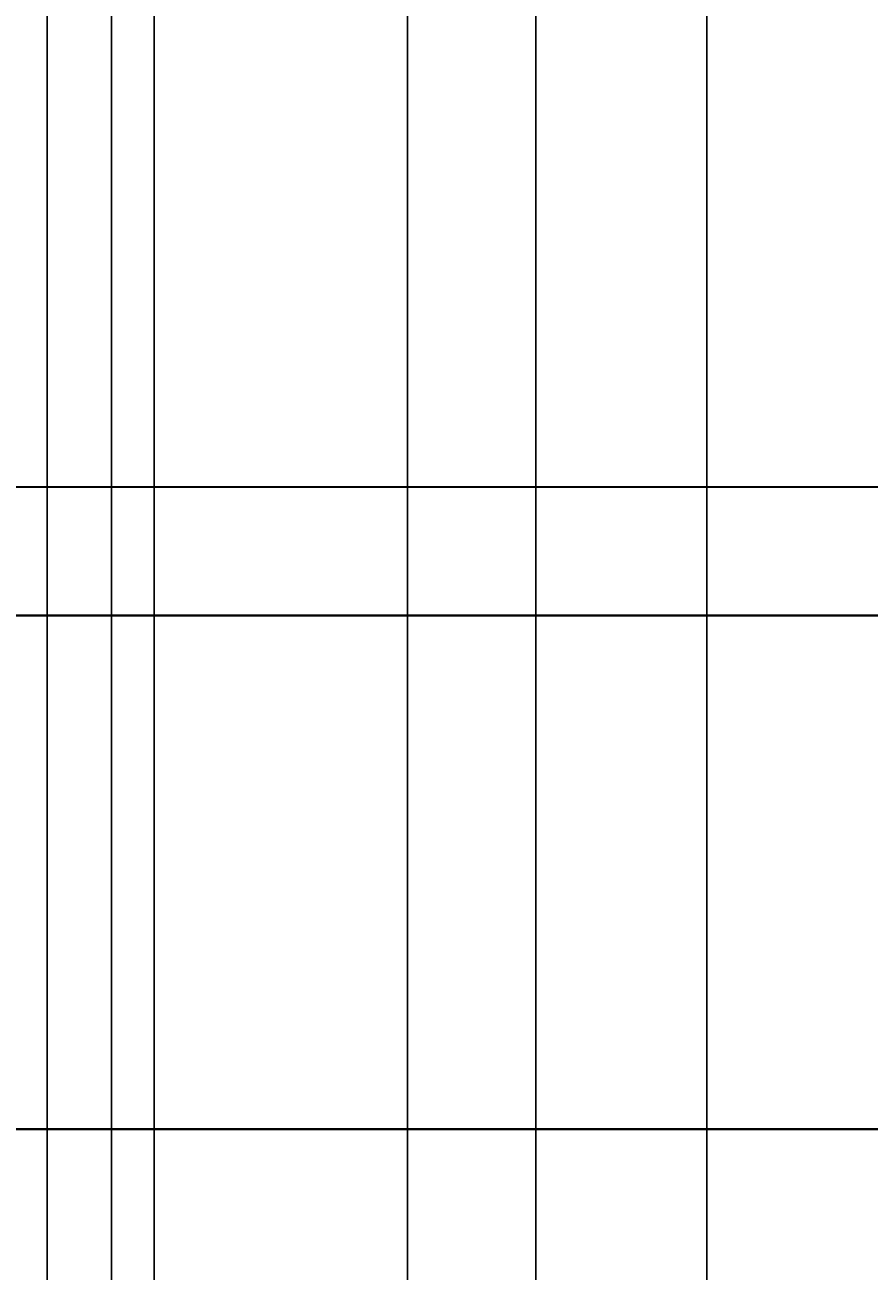
# Model space of a CAD drawing. Units: inches. Extents: x -6 to 289, y -8 to 323.
# Tile 49 of 107: x 126 to 146, y 124 to 153. Entities that reach past the tile are written whole.
import ezdxf

# ---------------------------------------------------------------- set-up
doc = ezdxf.new("R2010")
doc.units = ezdxf.units.IN
doc.header["$MEASUREMENT"] = 0
doc.layers.add('A-ANNO-DIMS', color=2, linetype='Continuous', lineweight=18)
doc.layers.add('A-ELEV', color=7, linetype='Continuous', lineweight=35)
doc.styles.get("Standard").update_dxf_attribs({"font": 'arial.ttf'})
doc.dimstyles.get("Standard").update_dxf_attribs({"dimtxt": 0.18, "dimasz": 0.18, "dimexe": 0.18, "dimexo": 0.0625, "dimgap": 0.09, "dimtad": 0, "dimtih": 1, "dimtoh": 1, "dimdec": 4, "dimzin": 0, "dimdsep": 46, "dimtxsty": 'Standard', "dimcen": 0.09, "dimadec": 0, "dimazin": 0, "dimtfac": 1, "dimtdec": 4, "dimtofl": 0, "dimtmove": 0, "dimatfit": 3, "dimfxl": 1, "dimtolj": 1, "dimtzin": 0, "dimarcsym": 0})

# ---------------------------------------------------------------- blocks, each defined once
blk = doc.blocks.new('*D24')
at = {"layer": 'A-ANNO-DIMS', "color": 0, "lineweight": -2, "transparency": 16777216}
for p, q in [((126.946, 178.654), (288.653, 178.654)), ((288.473, 178.474), (288.473, 159.153)), ((288.473, 139.469), (288.473, 158.789)), ((259.226, 139.289), (288.653, 139.289))]:
    blk.add_line(p, q, dxfattribs=at)
at = {"layer": 'A-ANNO-DIMS', "color": 0, "transparency": 16777216}
for points in [[(288.443, 178.474), (288.503, 178.474), (288.473, 178.654)], [(288.443, 139.469), (288.503, 139.469), (288.473, 139.289)]]:
    blk.add_solid(points, dxfattribs=at)
at = {"layer": 'Defpoints', "color": 0, "transparency": 16777216}
for p in [(126.883, 178.654), (288.473, 178.654), (259.164, 139.289)]:
    blk.add_point(p, dxfattribs=at)
at = {"layer": 'A-ANNO-DIMS', "color": 0, "transparency": 16777216, "insert": (288.473, 158.971), "char_height": 0.18, "attachment_point": 5}
blk.add_mtext('\\A1;39.365', dxfattribs=at)
blk = doc.blocks.new('*D28')
at = {"layer": 'A-ANNO-DIMS', "color": 0, "lineweight": -2, "transparency": 16777216}
for p, q in [((128.383, 180.092), (128.383, -8.391)), ((126.883, 178.592), (126.883, -8.391)), ((127.063, -8.211), (127.387, -8.211)), ((128.203, -8.211), (127.88, -8.211))]:
    blk.add_line(p, q, dxfattribs=at)
at = {"layer": 'A-ANNO-DIMS', "color": 0, "transparency": 16777216}
for points in [[(127.063, -8.181), (127.063, -8.241), (126.883, -8.211)], [(128.203, -8.181), (128.203, -8.241), (128.383, -8.211)]]:
    blk.add_solid(points, dxfattribs=at)
at = {"layer": 'Defpoints', "color": 0, "transparency": 16777216}
for p in [(128.383, 180.154), (126.883, 178.654), (128.383, -8.211)]:
    blk.add_point(p, dxfattribs=at)
at = {"layer": 'A-ANNO-DIMS', "color": 0, "transparency": 16777216, "insert": (127.633, -8.211), "char_height": 0.18, "attachment_point": 5}
blk.add_mtext('\\A1;1.5', dxfattribs=at)
blk = doc.blocks.new('*D29')
at = {"layer": 'A-ANNO-DIMS', "color": 0, "lineweight": -2, "transparency": 16777216}
for p, q in [((129.383, 181.092), (129.383, -8.391)), ((128.383, 180.092), (128.383, -8.391)), ((128.563, -8.211), (128.76, -8.211)), ((129.203, -8.211), (129.007, -8.211))]:
    blk.add_line(p, q, dxfattribs=at)
at = {"layer": 'A-ANNO-DIMS', "color": 0, "transparency": 16777216}
for points in [[(128.563, -8.181), (128.563, -8.241), (128.383, -8.211)], [(129.203, -8.181), (129.203, -8.241), (129.383, -8.211)]]:
    blk.add_solid(points, dxfattribs=at)
at = {"layer": 'Defpoints', "color": 0, "transparency": 16777216}
for p in [(129.383, 181.154), (128.383, 180.154), (129.383, -8.211)]:
    blk.add_point(p, dxfattribs=at)
at = {"layer": 'A-ANNO-DIMS', "color": 0, "transparency": 16777216, "insert": (128.883, -8.211), "char_height": 0.18, "attachment_point": 5}
blk.add_mtext('\\A1;1', dxfattribs=at)
blk = doc.blocks.new('*D30')
at = {"layer": 'A-ANNO-DIMS', "color": 0, "lineweight": -2, "transparency": 16777216}
for p, q in [((129.383, 181.092), (129.383, -8.391)), ((146.883, 181.092), (146.883, -8.391)), ((129.563, -8.211), (137.817, -8.211)), ((146.703, -8.211), (138.449, -8.211))]:
    blk.add_line(p, q, dxfattribs=at)
at = {"layer": 'A-ANNO-DIMS', "color": 0, "transparency": 16777216}
for points in [[(129.563, -8.181), (129.563, -8.241), (129.383, -8.211)], [(146.703, -8.181), (146.703, -8.241), (146.883, -8.211)]]:
    blk.add_solid(points, dxfattribs=at)
at = {"layer": 'Defpoints', "color": 0, "transparency": 16777216}
for p in [(129.383, 181.154), (146.883, 181.154), (146.883, -8.211)]:
    blk.add_point(p, dxfattribs=at)
at = {"layer": 'A-ANNO-DIMS', "color": 0, "transparency": 16777216, "insert": (138.133, -8.211), "char_height": 0.18, "attachment_point": 5}
blk.add_mtext('\\A1;17.5', dxfattribs=at)
blk = doc.blocks.new('*D73')
at = {"layer": 'A-ANNO-DIMS', "color": 0, "lineweight": -2, "transparency": 16777216}
for p, q in [((121.008, 51.148), (121.008, 322.969)), ((135.296, 51.148), (135.296, 322.969)), ((121.188, 322.789), (127.697, 322.789)), ((135.116, 322.789), (128.607, 322.789))]:
    blk.add_line(p, q, dxfattribs=at)
at = {"layer": 'A-ANNO-DIMS', "color": 0, "transparency": 16777216}
for points in [[(121.188, 322.819), (121.188, 322.759), (121.008, 322.789)], [(135.116, 322.819), (135.116, 322.759), (135.296, 322.789)]]:
    blk.add_solid(points, dxfattribs=at)
at = {"layer": 'Defpoints', "color": 0, "transparency": 16777216}
for p in [(135.296, 322.789), (121.008, 51.085), (135.296, 51.085)]:
    blk.add_point(p, dxfattribs=at)
at = {"layer": 'A-ANNO-DIMS', "color": 0, "transparency": 16777216, "insert": (128.152, 322.789), "char_height": 0.18, "attachment_point": 5}
blk.add_mtext('\\A1;14.288', dxfattribs=at)
blk = doc.blocks.new('*D74')
at = {"layer": 'A-ANNO-DIMS', "color": 0, "lineweight": -2, "transparency": 16777216}
for p, q in [((135.296, 51.148), (135.296, 322.969)), ((138.296, 51.148), (138.296, 322.969)), ((135.476, 322.789), (136.647, 322.789)), ((138.116, 322.789), (136.945, 322.789))]:
    blk.add_line(p, q, dxfattribs=at)
at = {"layer": 'A-ANNO-DIMS', "color": 0, "transparency": 16777216}
for points in [[(135.476, 322.819), (135.476, 322.759), (135.296, 322.789)], [(138.116, 322.819), (138.116, 322.759), (138.296, 322.789)]]:
    blk.add_solid(points, dxfattribs=at)
at = {"layer": 'Defpoints', "color": 0, "transparency": 16777216}
for p in [(138.296, 322.789), (135.296, 51.085), (138.296, 51.085)]:
    blk.add_point(p, dxfattribs=at)
at = {"layer": 'A-ANNO-DIMS', "color": 0, "transparency": 16777216, "insert": (136.796, 322.789), "char_height": 0.18, "attachment_point": 5}
blk.add_mtext('\\A1;3', dxfattribs=at)
blk = doc.blocks.new('*D75')
at = {"layer": 'A-ANNO-DIMS', "color": 0, "lineweight": -2, "transparency": 16777216}
for p, q in [((138.296, 51.148), (138.296, 322.969)), ((142.296, 51.148), (142.296, 322.969)), ((138.476, 322.789), (140.144, 322.789)), ((142.116, 322.789), (140.448, 322.789))]:
    blk.add_line(p, q, dxfattribs=at)
at = {"layer": 'A-ANNO-DIMS', "color": 0, "transparency": 16777216}
for points in [[(138.476, 322.819), (138.476, 322.759), (138.296, 322.789)], [(142.116, 322.819), (142.116, 322.759), (142.296, 322.789)]]:
    blk.add_solid(points, dxfattribs=at)
at = {"layer": 'Defpoints', "color": 0, "transparency": 16777216}
for p in [(142.296, 322.789), (138.296, 51.085), (142.296, 51.085)]:
    blk.add_point(p, dxfattribs=at)
at = {"layer": 'A-ANNO-DIMS', "color": 0, "transparency": 16777216, "insert": (140.296, 322.789), "char_height": 0.18, "attachment_point": 5}
blk.add_mtext('\\A1;4', dxfattribs=at)
blk = doc.blocks.new('*D76')
at = {"layer": 'A-ANNO-DIMS', "color": 0, "lineweight": -2, "transparency": 16777216}
for p, q in [((142.296, 51.148), (142.296, 322.969)), ((164.296, 51.148), (164.296, 322.969)), ((142.476, 322.789), (153.076, 322.789)), ((164.116, 322.789), (153.516, 322.789))]:
    blk.add_line(p, q, dxfattribs=at)
at = {"layer": 'A-ANNO-DIMS', "color": 0, "transparency": 16777216}
for points in [[(142.476, 322.819), (142.476, 322.759), (142.296, 322.789)], [(164.116, 322.819), (164.116, 322.759), (164.296, 322.789)]]:
    blk.add_solid(points, dxfattribs=at)
at = {"layer": 'Defpoints', "color": 0, "transparency": 16777216}
for p in [(164.296, 322.789), (142.296, 51.085), (164.296, 51.085)]:
    blk.add_point(p, dxfattribs=at)
at = {"layer": 'A-ANNO-DIMS', "color": 0, "transparency": 16777216, "insert": (153.296, 322.789), "char_height": 0.18, "attachment_point": 5}
blk.add_mtext('\\A1;22', dxfattribs=at)

msp = doc.modelspace()

# ---------------------------------------------------------------- linework, layer by layer
at = {"layer": 'A-ELEV'}
for p, q in [((115.1638, 139.2888), (259.1638, 139.2888)), ((259.1638, 127.2888), (115.1638, 127.2888)), ((115.1638, 127.2888), (259.1638, 127.2888))]:
    msp.add_line(p, q, dxfattribs=at)
for points in [[(247.1638, 139.2888), (115.1638, 139.2888), (115.1638, 162.3484), (247.1638, 162.3484)], [(244.1638, 142.2888), (118.1638, 142.2888), (118.1638, 159.3484), (244.1638, 159.3484)]]:
    msp.add_lwpolyline(points, close=True, dxfattribs=at)

# ---------------------------------------------------------------- dimensions: what is measured, and where the dimension line sits
at = {"layer": 'A-ANNO-DIMS'}
for base, p1, p2, override, picture, middle in [((135.296, 322.7888), (121.008, 51.0851), (135.296, 51.0851), {"dimdec": 3, "dimlfac": 1, "dimrnd": 0, "dimzin": 0, "dimdsep": 46, "dimlunit": 2}, '*D73', (128.152, 322.7888)), ((138.296, 322.7888), (135.296, 51.0851), (138.296, 51.0851), {"dimdec": 0, "dimlfac": 1, "dimrnd": 0, "dimzin": 0, "dimdsep": 46, "dimlunit": 2}, '*D74', (136.796, 322.7888)), ((142.296, 322.7888), (138.296, 51.0851), (142.296, 51.0851), {"dimdec": 0, "dimlfac": 1, "dimrnd": 0, "dimzin": 0, "dimdsep": 46, "dimlunit": 2}, '*D75', (140.296, 322.7888)), ((164.296, 322.7888), (142.296, 51.0851), (164.296, 51.0851), {"dimdec": 0, "dimlfac": 1, "dimrnd": 0, "dimzin": 0, "dimdsep": 46, "dimlunit": 2}, '*D76', (153.296, 322.7888)), ((129.3835, -8.2112), (128.3835, 180.154), (129.3835, 181.154), {"dimdec": 0, "dimlfac": 1, "dimrnd": 0, "dimzin": 0, "dimdsep": 46, "dimlunit": 2}, '*D29', (128.8835, -8.2112)), ((146.8835, -8.2112), (129.3835, 181.154), (146.8835, 181.154), {"dimdec": 1, "dimlfac": 1, "dimrnd": 0, "dimzin": 0, "dimdsep": 46, "dimlunit": 2}, '*D30', (138.1335, -8.2112)), ((128.3835, -8.2112), (126.8835, 178.654), (128.3835, 180.154), {"dimdec": 1, "dimlfac": 1, "dimrnd": 0, "dimzin": 0, "dimdsep": 46, "dimlunit": 2}, '*D28', (127.6335, -8.2112))]:
    dim = msp.add_linear_dim(base=base, p1=p1, p2=p2, dimstyle='Standard', override=override, dxfattribs=at)
    dim.commit()
    dim.dimension.update_dxf_attribs({"geometry": picture, "text_midpoint": middle})
dim = msp.add_linear_dim(base=(288.4733, 178.654), p1=(259.1638, 139.2888), p2=(126.8835, 178.654), angle=90, dimstyle='Standard', override={"dimdec": 3, "dimlfac": 1, "dimrnd": 0, "dimzin": 0, "dimdsep": 46, "dimlunit": 2}, dxfattribs=at)
dim.commit()
dim.dimension.update_dxf_attribs({"geometry": '*D24', "text_midpoint": (288.4733, 158.9714)})

doc.saveas('drawing.dxf')
